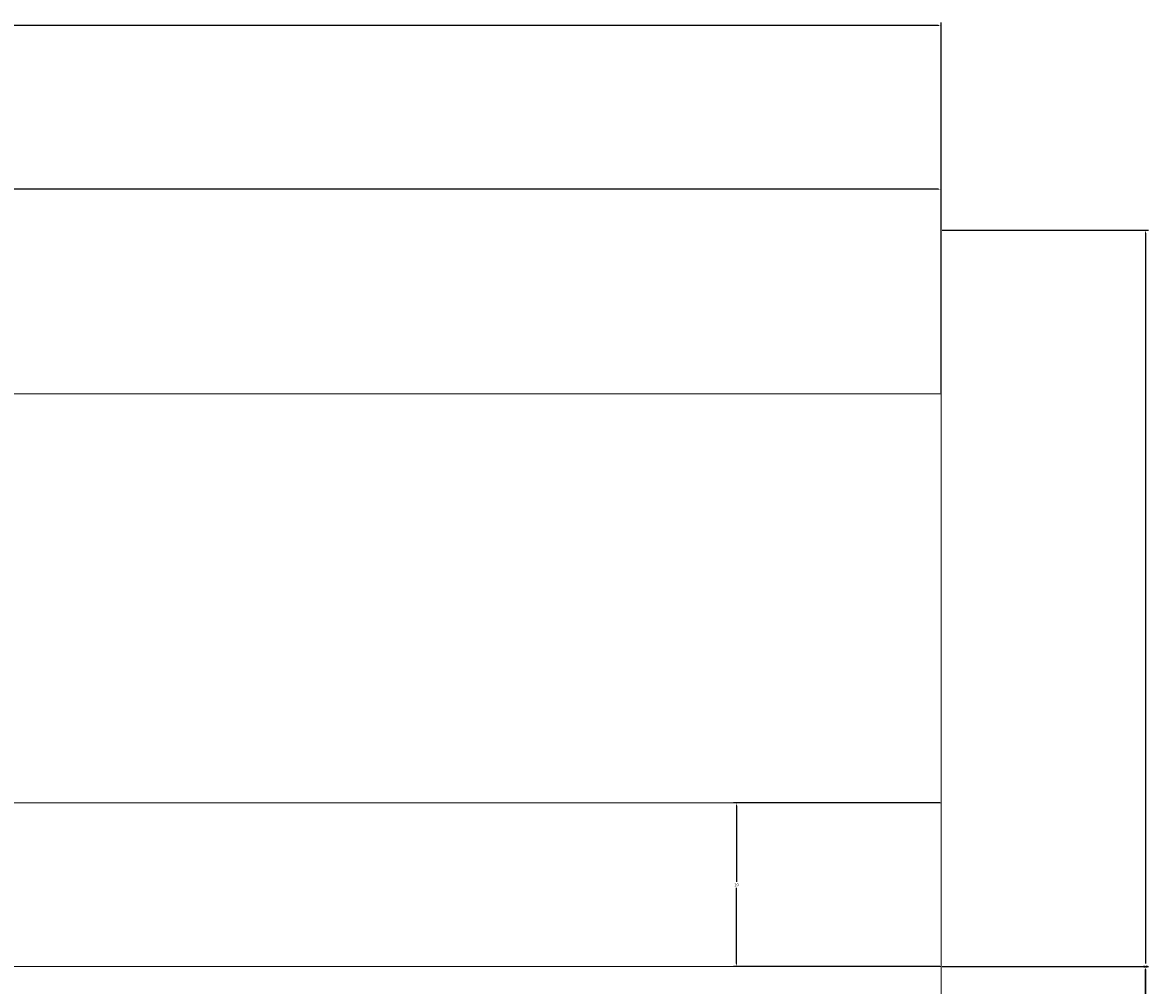
# Model space of a CAD drawing. Units: millimetres. Extents: x 135 to 361, y -58 to 58.
# Tile 5 of 5: x 292 to 361, y -1 to 58. Entities that reach past the tile are written whole.
import ezdxf

# ---------------------------------------------------------------- set-up
doc = ezdxf.new("R2010")
doc.units = ezdxf.units.MM
doc.layers.add('M-CONS', color=8, linetype='Continuous', lineweight=13)
doc.layers.add('M-DIMS', color=2, linetype='Continuous', lineweight=18)
doc.styles.get("Standard").update_dxf_attribs({"font": 'arial.ttf'})
doc.dimstyles.get("Standard").update_dxf_attribs({"dimtxt": 0.18, "dimasz": 0.18, "dimexe": 0.18, "dimexo": 0.0625, "dimgap": 0.09, "dimtad": 0, "dimtih": 1, "dimtoh": 1, "dimdec": 4, "dimzin": 0, "dimdsep": 46, "dimtxsty": 'Standard', "dimcen": 0.09, "dimadec": 0, "dimazin": 0, "dimtfac": 1, "dimtdec": 4, "dimtofl": 0, "dimtmove": 0, "dimatfit": 3, "dimfxl": 1, "dimtolj": 1, "dimtzin": 0, "dimarcsym": 0})

# ---------------------------------------------------------------- blocks, each defined once
blk = doc.blocks.new('*D1')
at = {"layer": 'Defpoints', "color": 0, "transparency": 16777216}
for p in [(347.813, 57.5), (347.813, 45), (147.813, 35)]:
    blk.add_point(p, dxfattribs=at)
at = {"layer": 'M-DIMS', "color": 0, "lineweight": -2, "transparency": 16777216}
for p, q in [((147.813, 35.062), (147.813, 57.68)), ((147.993, 57.5), (247.522, 57.5)), ((347.633, 57.5), (248.103, 57.5)), ((347.813, 45.062), (347.813, 57.68))]:
    blk.add_line(p, q, dxfattribs=at)
at = {"layer": 'M-DIMS', "color": 0, "transparency": 16777216}
for points in [[(147.993, 57.53), (147.993, 57.47), (147.813, 57.5)], [(347.633, 57.53), (347.633, 57.47), (347.813, 57.5)]]:
    blk.add_solid(points, dxfattribs=at)
at = {"layer": 'M-DIMS', "color": 0, "transparency": 16777216, "insert": (247.813, 57.5), "char_height": 0.18, "attachment_point": 5}
blk.add_mtext('\\A1;200', dxfattribs=at)
blk = doc.blocks.new('*D2')
at = {"layer": 'Defpoints', "color": 0, "transparency": 16777216}
for p in [(347.813, 45), (347.813, -45), (360.313, -45)]:
    blk.add_point(p, dxfattribs=at)
at = {"layer": 'M-DIMS', "color": 0, "lineweight": -2, "transparency": 16777216}
for p, q in [((347.875, 45), (360.493, 45)), ((360.313, 44.82), (360.313, 0.182)), ((360.313, -44.82), (360.313, -0.182)), ((347.875, -45), (360.493, -45))]:
    blk.add_line(p, q, dxfattribs=at)
at = {"layer": 'M-DIMS', "color": 0, "transparency": 16777216}
for points in [[(360.283, 44.82), (360.343, 44.82), (360.313, 45)], [(360.283, -44.82), (360.343, -44.82), (360.313, -45)]]:
    blk.add_solid(points, dxfattribs=at)
at = {"layer": 'M-DIMS', "color": 0, "transparency": 16777216, "insert": (360.313, 0), "char_height": 0.18, "attachment_point": 5}
blk.add_mtext('\\A1;90', dxfattribs=at)
blk = doc.blocks.new('*D3')
at = {"layer": 'Defpoints', "color": 0, "transparency": 16777216}
for p in [(347.813, 47.5), (222.813, 35), (347.813, 35)]:
    blk.add_point(p, dxfattribs=at)
at = {"layer": 'M-DIMS', "color": 0, "lineweight": -2, "transparency": 16777216}
for p, q in [((222.813, 35.062), (222.813, 47.68)), ((347.813, 35.062), (347.813, 47.68)), ((222.993, 47.5), (285.031, 47.5)), ((347.633, 47.5), (285.594, 47.5))]:
    blk.add_line(p, q, dxfattribs=at)
at = {"layer": 'M-DIMS', "color": 0, "transparency": 16777216}
for points in [[(222.993, 47.53), (222.993, 47.47), (222.813, 47.5)], [(347.633, 47.53), (347.633, 47.47), (347.813, 47.5)]]:
    blk.add_solid(points, dxfattribs=at)
at = {"layer": 'M-DIMS', "color": 0, "transparency": 16777216, "insert": (285.313, 47.5), "char_height": 0.18, "attachment_point": 5}
blk.add_mtext('\\A1;125', dxfattribs=at)
blk = doc.blocks.new('*D5')
at = {"layer": 'Defpoints', "color": 0, "transparency": 16777216}
for p in [(335.313, 10), (347.813, 10), (347.813, 0)]:
    blk.add_point(p, dxfattribs=at)
at = {"layer": 'M-DIMS', "color": 0, "lineweight": -2, "transparency": 16777216}
for p, q in [((347.75, 10), (335.133, 10)), ((335.313, 9.82), (335.313, 5.182)), ((335.313, 0.18), (335.313, 4.818)), ((347.75, 0), (335.133, 0))]:
    blk.add_line(p, q, dxfattribs=at)
at = {"layer": 'M-DIMS', "color": 0, "transparency": 16777216}
for points in [[(335.283, 9.82), (335.343, 9.82), (335.313, 10)], [(335.283, 0.18), (335.343, 0.18), (335.313, 0)]]:
    blk.add_solid(points, dxfattribs=at)
at = {"layer": 'M-DIMS', "color": 0, "transparency": 16777216, "insert": (335.313, 5), "char_height": 0.18, "attachment_point": 5}
blk.add_mtext('\\A1;10', dxfattribs=at)
blk = doc.blocks.new('*D9')
at = {"layer": 'Defpoints', "color": 0, "transparency": 16777216}
for p in [(347.813, 0), (360.313, 0), (302.813, -22.5)]:
    blk.add_point(p, dxfattribs=at)
at = {"layer": 'M-DIMS', "color": 0, "lineweight": -2, "transparency": 16777216}
for p, q in [((347.875, 0), (360.493, 0)), ((360.313, -0.18), (360.313, -11.068)), ((360.313, -22.32), (360.313, -11.432)), ((302.875, -22.5), (360.493, -22.5))]:
    blk.add_line(p, q, dxfattribs=at)
at = {"layer": 'M-DIMS', "color": 0, "transparency": 16777216}
for points in [[(360.283, -0.18), (360.343, -0.18), (360.313, 0)], [(360.283, -22.32), (360.343, -22.32), (360.313, -22.5)]]:
    blk.add_solid(points, dxfattribs=at)
at = {"layer": 'M-DIMS', "color": 0, "transparency": 16777216, "insert": (360.313, -11.25), "char_height": 0.18, "attachment_point": 5}
blk.add_mtext('\\A1;22.5', dxfattribs=at)

msp = doc.modelspace()

# ---------------------------------------------------------------- linework, layer by layer
at = {"layer": 'M-CONS', "extrusion": (0, -1, 0)}
msp.add_line((347.813, 0, 117.744), (347.813, 45, 117.744), dxfattribs=at)
at = {"layer": 'M-CONS', "elevation": 93.744}
for points in [[(347.813, 10), (347.813, 35), (222.813, 35), (222.813, 10)], [(347.813, -45), (257.813, -45), (257.813, 0), (347.813, 0)]]:
    msp.add_lwpolyline(points, close=True, dxfattribs=at)
at = {"layer": 'M-CONS', "extrusion": (0, -1, 0)}
msp.add_lwpolyline([(167.813, 133.744), (284.813, 145.744), (347.813, 117.744), (347.813, 93.744), (167.813, 93.744)], dxfattribs=at)

# ---------------------------------------------------------------- dimensions: what is measured, and where the dimension line sits
at = {"layer": 'M-DIMS'}
for base, p1, p2, picture, middle in [((347.813, 57.5), (147.813, 35), (347.813, 45), '*D1', (247.813, 57.5)), ((347.813, 47.5), (222.813, 35), (347.813, 35), '*D3', (285.313, 47.5))]:
    dim = msp.add_linear_dim(base=base, p1=p1, p2=p2, dimstyle='Standard', override={"dimdec": 0, "dimlfac": 1, "dimrnd": 0, "dimzin": 0, "dimdsep": 46, "dimlunit": 2}, dxfattribs=at)
    dim.commit()
    dim.dimension.update_dxf_attribs({"geometry": picture, "text_midpoint": middle})
for base, p1, p2, angle, override, picture, middle in [((360.313, -45), (347.813, 45), (347.813, -45), 270, {"dimdec": 0, "dimlfac": 1, "dimrnd": 0, "dimzin": 0, "dimdsep": 46, "dimlunit": 2}, '*D2', (360.313, 0)), ((335.313, 10), (347.813, 0), (347.813, 10), 90, {"dimdec": 0, "dimlfac": 1, "dimrnd": 0, "dimzin": 0, "dimdsep": 46, "dimlunit": 2}, '*D5', (335.313, 5)), ((360.313, 0), (302.813, -22.5), (347.813, 0), 90, {"dimdec": 1, "dimlfac": 1, "dimrnd": 0, "dimzin": 0, "dimdsep": 46, "dimlunit": 2}, '*D9', (360.313, -11.25))]:
    dim = msp.add_linear_dim(base=base, p1=p1, p2=p2, angle=angle, dimstyle='Standard', override=override, dxfattribs=at)
    dim.commit()
    dim.dimension.update_dxf_attribs({"geometry": picture, "text_midpoint": middle})

doc.saveas('drawing.dxf')
